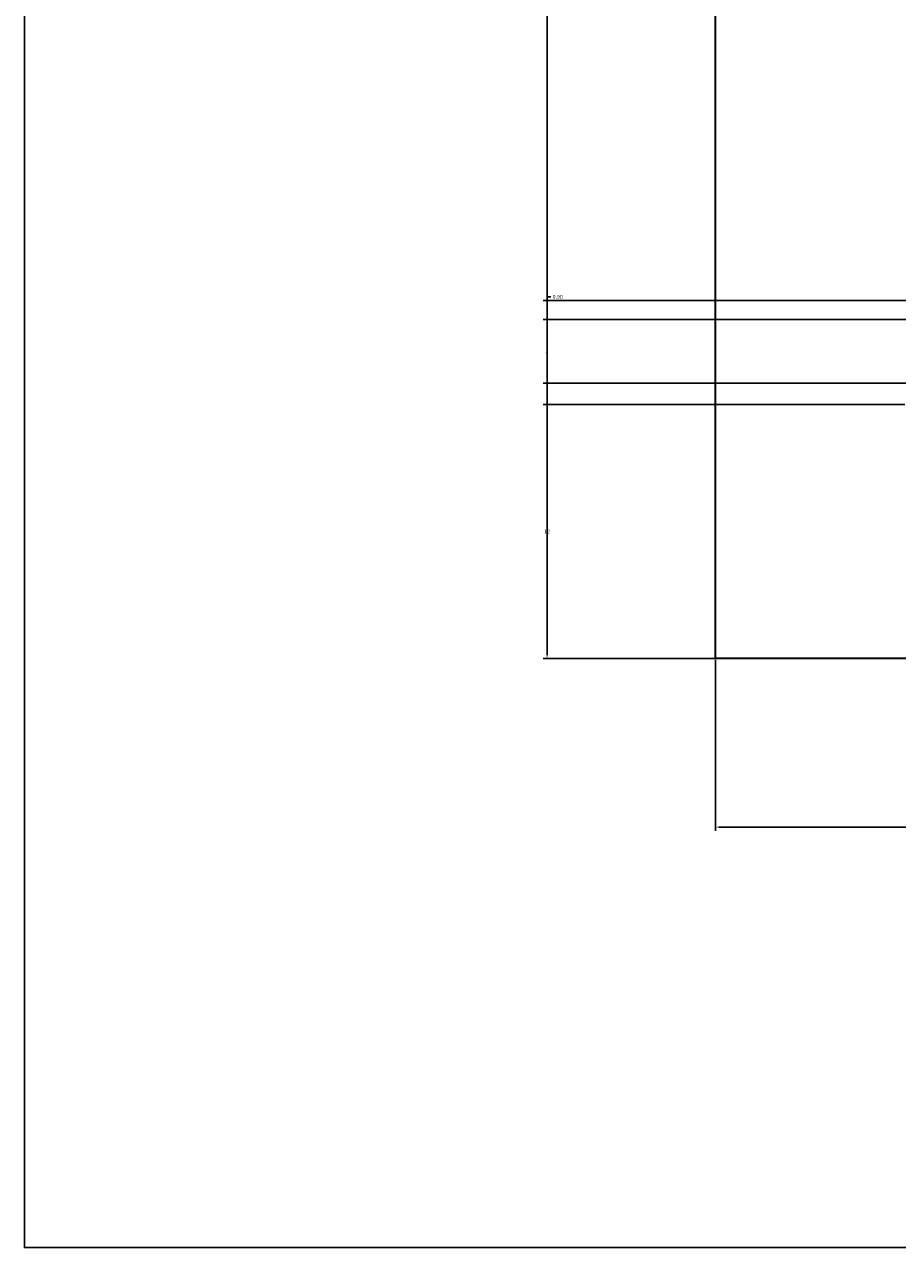
# Model space of a CAD drawing. Units: inches. Extents: x 4508 to 4723, y 847 to 1020.
# Tile 1 of 32: x 4508 to 4550, y 847 to 905. Entities that reach past the tile are written whole.
import ezdxf

# ---------------------------------------------------------------- set-up
doc = ezdxf.new("R2010")
doc.units = ezdxf.units.IN
for name, color, linetype, lineweight in [('A-ANNO-DIMS', 2, 'Continuous', 18), ('A-ANNO-TTLB', 7, 'Continuous', 25), ('A-WALL', 7, 'Continuous', 35)]:
    doc.layers.add(name, color=color, linetype=linetype, lineweight=lineweight)
doc.styles.get("Standard").update_dxf_attribs({"font": 'arial.ttf'})
doc.dimstyles.get("Standard").update_dxf_attribs({"dimtxt": 0.18, "dimasz": 0.18, "dimexe": 0.18, "dimexo": 0.0625, "dimgap": 0.09, "dimtad": 0, "dimtih": 1, "dimtoh": 1, "dimdec": 4, "dimzin": 0, "dimdsep": 46, "dimtxsty": 'Standard', "dimcen": 0.09, "dimadec": 0, "dimazin": 0, "dimtfac": 1, "dimtdec": 4, "dimtofl": 0, "dimtmove": 0, "dimatfit": 3, "dimfxl": 1, "dimtolj": 1, "dimtzin": 0, "dimarcsym": 0})

# ---------------------------------------------------------------- blocks, each defined once
blk = doc.blocks.new('*D2')
at = {"layer": 'A-ANNO-DIMS', "color": 0, "lineweight": -2, "transparency": 16777216}
for p, q in [((4540.994, 874.684), (4540.994, 866.617)), ((4693.994, 874.684), (4693.994, 866.617)), ((4541.174, 866.797), (4617.213, 866.797)), ((4693.814, 866.797), (4617.774, 866.797))]:
    blk.add_line(p, q, dxfattribs=at)
at = {"layer": 'A-ANNO-DIMS', "color": 0, "lineweight": 9, "transparency": 16777216}
for points in [[(4541.174, 866.827), (4541.174, 866.767), (4540.994, 866.797)], [(4693.814, 866.827), (4693.814, 866.767), (4693.994, 866.797)]]:
    blk.add_solid(points, dxfattribs=at)
at = {"layer": 'Defpoints', "color": 0, "lineweight": 9, "transparency": 16777216}
for p in [(4540.994, 874.747), (4693.994, 874.747), (4693.994, 866.797)]:
    blk.add_point(p, dxfattribs=at)
at = {"layer": 'A-ANNO-DIMS', "color": 0, "transparency": 16777216, "insert": (4617.494, 866.797), "char_height": 0.18, "attachment_point": 5}
blk.add_mtext('\\A1;153', dxfattribs=at)
blk = doc.blocks.new('*D3')
at = {"layer": 'A-ANNO-DIMS', "color": 0, "lineweight": -2, "transparency": 16777216}
for p, q in [((4540.931, 994.747), (4532.864, 994.747)), ((4533.044, 994.567), (4533.044, 934.929)), ((4533.044, 874.927), (4533.044, 934.565)), ((4540.931, 874.747), (4532.864, 874.747))]:
    blk.add_line(p, q, dxfattribs=at)
at = {"layer": 'A-ANNO-DIMS', "color": 0, "lineweight": 9, "transparency": 16777216}
for points in [[(4533.014, 994.567), (4533.074, 994.567), (4533.044, 994.747)], [(4533.014, 874.927), (4533.074, 874.927), (4533.044, 874.747)]]:
    blk.add_solid(points, dxfattribs=at)
at = {"layer": 'Defpoints', "color": 0, "lineweight": 9, "transparency": 16777216}
for p in [(4533.044, 994.747), (4540.994, 994.747), (4540.994, 874.747)]:
    blk.add_point(p, dxfattribs=at)
at = {"layer": 'A-ANNO-DIMS', "color": 0, "transparency": 16777216, "insert": (4533.044, 934.747), "char_height": 0.18, "attachment_point": 5}
blk.add_mtext('\\A1;120', dxfattribs=at)
blk = doc.blocks.new('*D14')
at = {"layer": 'A-ANNO-DIMS', "color": 0, "lineweight": -2, "transparency": 16777216}
for p, q in [((4549.931, 886.747), (4532.864, 886.747)), ((4533.044, 886.567), (4533.044, 880.927)), ((4533.044, 874.927), (4533.044, 880.567)), ((4549.931, 874.747), (4532.864, 874.747))]:
    blk.add_line(p, q, dxfattribs=at)
at = {"layer": 'A-ANNO-DIMS', "color": 0, "lineweight": 9, "transparency": 16777216}
for points in [[(4533.014, 886.567), (4533.074, 886.567), (4533.044, 886.747)], [(4533.014, 874.927), (4533.074, 874.927), (4533.044, 874.747)]]:
    blk.add_solid(points, dxfattribs=at)
at = {"layer": 'Defpoints', "color": 0, "lineweight": 9, "transparency": 16777216}
for p in [(4533.044, 886.747), (4549.994, 886.747), (4549.994, 874.747)]:
    blk.add_point(p, dxfattribs=at)
at = {"layer": 'A-ANNO-DIMS', "color": 0, "transparency": 16777216, "insert": (4533.044, 880.747), "char_height": 0.18, "attachment_point": 5}
blk.add_mtext('\\A1;12', dxfattribs=at)
blk = doc.blocks.new('*D32')
at = {"layer": 'A-ANNO-DIMS', "color": 0, "lineweight": -2, "transparency": 16777216}
for p, q in [((4604.431, 890.747), (4532.864, 890.747)), ((4533.044, 890.567), (4533.044, 889.429)), ((4533.044, 887.927), (4533.044, 889.065)), ((4604.431, 887.747), (4532.864, 887.747))]:
    blk.add_line(p, q, dxfattribs=at)
at = {"layer": 'A-ANNO-DIMS', "color": 0, "lineweight": 9, "transparency": 16777216}
for points in [[(4533.014, 890.567), (4533.074, 890.567), (4533.044, 890.747)], [(4533.014, 887.927), (4533.074, 887.927), (4533.044, 887.747)]]:
    blk.add_solid(points, dxfattribs=at)
at = {"layer": 'Defpoints', "color": 0, "lineweight": 9, "transparency": 16777216}
for p in [(4533.044, 890.747), (4604.494, 890.747), (4604.494, 887.747)]:
    blk.add_point(p, dxfattribs=at)
at = {"layer": 'A-ANNO-DIMS', "color": 0, "transparency": 16777216, "insert": (4533.044, 889.247), "char_height": 0.18, "attachment_point": 5}
blk.add_mtext('\\A1;3', dxfattribs=at)
blk = doc.blocks.new('*D41')
at = {"layer": 'A-ANNO-DIMS', "color": 0, "lineweight": -2, "transparency": 16777216}
for p, q in [((4533.044, 891.643), (4533.044, 891.823)), ((4533.044, 891.823), (4533.224, 891.823)), ((4616.47, 891.643), (4532.864, 891.643)), ((4533.044, 890.927), (4533.044, 891.463)), ((4608.499, 890.747), (4532.864, 890.747))]:
    blk.add_line(p, q, dxfattribs=at)
at = {"layer": 'A-ANNO-DIMS', "color": 0, "lineweight": 9, "transparency": 16777216}
for points in [[(4533.014, 891.463), (4533.074, 891.463), (4533.044, 891.643)], [(4533.014, 890.927), (4533.074, 890.927), (4533.044, 890.747)]]:
    blk.add_solid(points, dxfattribs=at)
at = {"layer": 'Defpoints', "color": 0, "lineweight": 9, "transparency": 16777216}
for p in [(4533.044, 891.643), (4616.533, 891.643), (4608.562, 890.747)]:
    blk.add_point(p, dxfattribs=at)
at = {"layer": 'A-ANNO-DIMS', "color": 0, "transparency": 16777216, "insert": (4533.547, 891.823), "char_height": 0.18, "attachment_point": 5}
blk.add_mtext('\\A1;0.90', dxfattribs=at)

msp = doc.modelspace()

# ---------------------------------------------------------------- linework, layer by layer
at = {"layer": 'A-ANNO-TTLB'}
msp.add_lwpolyline([(4508.3867, 1019.9118), (4722.9774, 1019.9118), (4722.9774, 846.9535), (4508.3867, 846.9535)], close=True, dxfattribs=at)
at = {"layer": 'A-WALL'}
for p, q in [((4540.9938, 874.7469), (4540.9938, 994.7469)), ((4549.9938, 874.7469), (4540.9938, 874.7469))]:
    msp.add_line(p, q, dxfattribs=at)

# ---------------------------------------------------------------- dimensions: what is measured, and where the dimension line sits
at = {"layer": 'A-ANNO-DIMS'}
for base, p1, p2, override, picture, middle in [((4533.0438, 994.7469), (4540.9938, 874.7469), (4540.9938, 994.7469), {"dimdec": 0, "dimlfac": 1, "dimrnd": 0, "dimzin": 0, "dimdsep": 46, "dimlunit": 2}, '*D3', (4533.0438, 934.7469)), ((4533.0438, 891.6433), (4608.5617, 890.7469), (4616.5328, 891.6433), {"dimdec": 2, "dimlfac": 1, "dimrnd": 0, "dimzin": 0, "dimdsep": 46, "dimlunit": 2}, '*D41', (4533.5473, 891.8233)), ((4533.0438, 890.7469), (4604.4938, 887.7469), (4604.4938, 890.7469), {"dimdec": 0, "dimlfac": 1, "dimrnd": 0, "dimzin": 0, "dimdsep": 46, "dimlunit": 2}, '*D32', (4533.0438, 889.2469)), ((4533.0438, 886.7469), (4549.9938, 874.7469), (4549.9938, 886.7469), {"dimdec": 0, "dimlfac": 1, "dimrnd": 0, "dimzin": 0, "dimdsep": 46, "dimlunit": 2}, '*D14', (4533.0438, 880.7469))]:
    dim = msp.add_linear_dim(base=base, p1=p1, p2=p2, angle=90, dimstyle='Standard', override=override, dxfattribs=at)
    dim.commit()
    dim.dimension.update_dxf_attribs({"geometry": picture, "text_midpoint": middle})
dim = msp.add_linear_dim(base=(4693.9938, 866.7969), p1=(4540.9938, 874.7469), p2=(4693.9938, 874.7469), dimstyle='Standard', override={"dimdec": 0, "dimlfac": 1, "dimrnd": 0, "dimzin": 0, "dimdsep": 46, "dimlunit": 2}, dxfattribs=at)
dim.commit()
dim.dimension.update_dxf_attribs({"geometry": '*D2', "text_midpoint": (4617.4938, 866.7969)})

doc.saveas('drawing.dxf')
